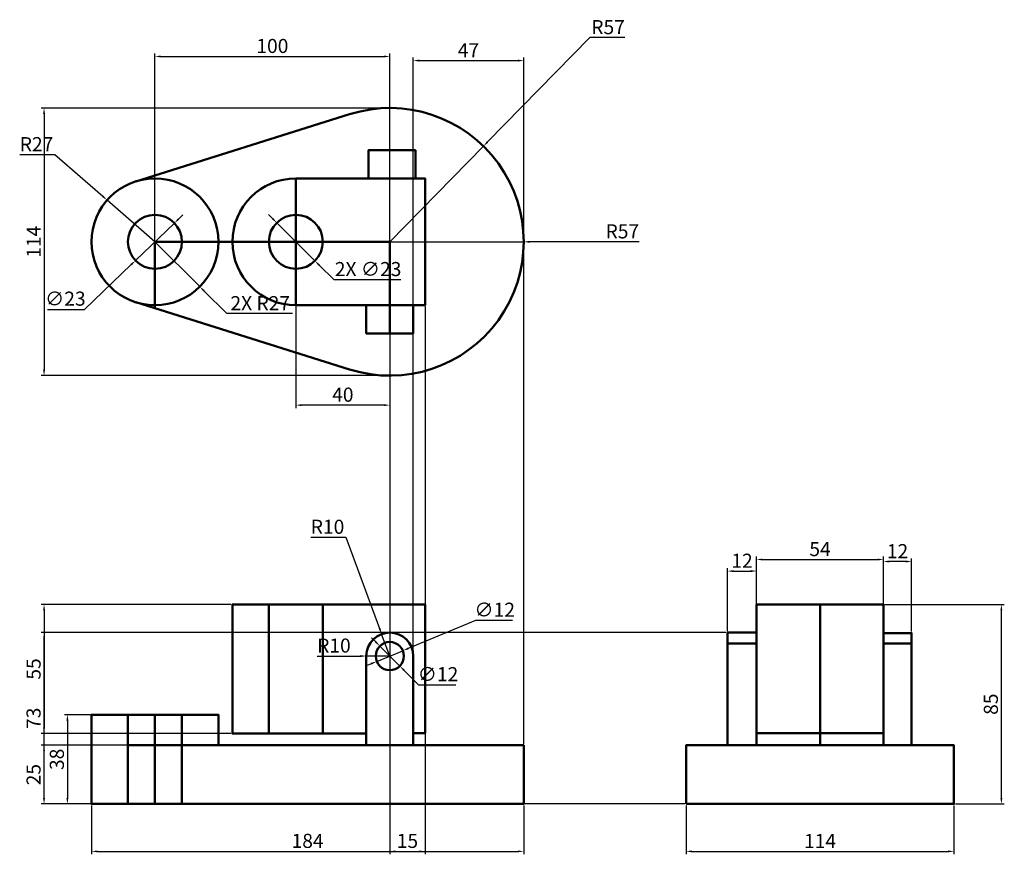
# Model space of a CAD drawing. Units: millimetres. Extents: x 186 to 605, y 16 to 372.
import ezdxf

# ---------------------------------------------------------------- set-up
doc = ezdxf.new("R2010")
doc.units = ezdxf.units.MM
doc.linetypes.add('CENTER', pattern=[50.8, 31.75, -6.35, 6.35, -6.35])
for name, color, linetype, lineweight in [('M-CNTR', 1, 'CENTER', 18), ('M-DIMS', 2, 'Continuous', 25), ('M-OUTL', 7, 'Continuous', 50)]:
    doc.layers.add(name, color=color, linetype=linetype, lineweight=lineweight)
doc.styles.get("Standard").update_dxf_attribs({"font": 'arial.ttf'})
doc.dimstyles.new('ISO-25', dxfattribs={"dimtxt": 6, "dimasz": 2.5, "dimexe": 1.25, "dimexo": 0.625, "dimtad": 1, "dimtoh": 1, "dimdec": 0, "dimtxsty": 'Standard', "dimcen": 2.5, "dimadec": 0, "dimazin": 0, "dimtfac": 1, "dimtdec": 0, "dimtmove": 0, "dimatfit": 3, "dimfxl": 1, "dimarcsym": 0})

# ---------------------------------------------------------------- blocks, each defined once
blk = doc.blocks.new('*D1')
at = {"layer": 'Defpoints', "color": 0, "transparency": 16777216}
for p in [(382.96, 318), (343.1, 277.26)]:
    blk.add_point(p, dxfattribs=at)
at = {"layer": 'M-DIMS', "color": 0, "lineweight": -2, "transparency": 16777216}
for p, q in [((428.23, 364.27), (384.71, 319.79)), ((443.19, 364.27), (428.23, 364.27)), ((343.1, 277.26), (382.96, 318))]:
    blk.add_line(p, q, dxfattribs=at)
at = {"layer": 'M-DIMS', "color": 0, "transparency": 16777216}
blk.add_solid([(384.41, 320.08), (385.01, 319.5), (382.96, 318)], dxfattribs=at)
at = {"layer": 'M-DIMS', "color": 0, "transparency": 16777216, "insert": (436.02, 367.94), "char_height": 6, "attachment_point": 5}
blk.add_mtext('R57', dxfattribs=at)
blk = doc.blocks.new('*D2')
at = {"layer": 'Defpoints', "color": 0, "transparency": 16777216}
for p in [(303.1, 277.26), (343.1, 277.26), (303.1, 207.7)]:
    blk.add_point(p, dxfattribs=at)
at = {"layer": 'M-DIMS', "color": 0, "lineweight": -2, "transparency": 16777216}
for p, q in [((303.1, 276.64), (303.1, 206.45)), ((343.1, 276.64), (343.1, 206.45)), ((340.6, 207.7), (305.6, 207.7))]:
    blk.add_line(p, q, dxfattribs=at)
at = {"layer": 'M-DIMS', "color": 0, "transparency": 16777216}
for points in [[(305.6, 208.12), (305.6, 207.28), (303.1, 207.7)], [(340.6, 208.12), (340.6, 207.28), (343.1, 207.7)]]:
    blk.add_solid(points, dxfattribs=at)
at = {"layer": 'M-DIMS', "color": 0, "transparency": 16777216, "insert": (323.1, 211.39), "char_height": 6, "attachment_point": 5}
blk.add_mtext('40', dxfattribs=at)
blk = doc.blocks.new('*D3')
at = {"layer": 'Defpoints', "color": 0, "transparency": 16777216}
for p in [(343.1, 356.22), (243.1, 277.26), (343.1, 277.26)]:
    blk.add_point(p, dxfattribs=at)
at = {"layer": 'M-DIMS', "color": 0, "lineweight": -2, "transparency": 16777216}
for p, q in [((243.1, 277.89), (243.1, 357.47)), ((343.1, 277.89), (343.1, 357.47)), ((245.6, 356.22), (340.6, 356.22))]:
    blk.add_line(p, q, dxfattribs=at)
at = {"layer": 'M-DIMS', "color": 0, "transparency": 16777216}
for points in [[(245.6, 356.64), (245.6, 355.8), (243.1, 356.22)], [(340.6, 356.64), (340.6, 355.8), (343.1, 356.22)]]:
    blk.add_solid(points, dxfattribs=at)
at = {"layer": 'M-DIMS', "color": 0, "transparency": 16777216, "insert": (293.1, 359.91), "char_height": 6, "attachment_point": 5}
blk.add_mtext('100', dxfattribs=at)
blk = doc.blocks.new('*D4')
at = {"layer": 'Defpoints', "color": 0, "transparency": 16777216}
for p in [(222.75, 295.01), (243.1, 277.26)]:
    blk.add_point(p, dxfattribs=at)
at = {"layer": 'M-DIMS', "color": 0, "lineweight": -2, "transparency": 16777216}
for p, q in [((185.53, 314.44), (200.49, 314.44)), ((200.49, 314.44), (220.87, 296.66)), ((243.1, 277.26), (222.75, 295.01))]:
    blk.add_line(p, q, dxfattribs=at)
at = {"layer": 'M-DIMS', "color": 0, "transparency": 16777216}
blk.add_solid([(221.14, 296.97), (220.6, 296.34), (222.75, 295.01)], dxfattribs=at)
at = {"layer": 'M-DIMS', "color": 0, "transparency": 16777216, "insert": (192.7, 318.08), "char_height": 6, "attachment_point": 5}
blk.add_mtext('R27', dxfattribs=at)
blk = doc.blocks.new('*D5')
at = {"layer": 'Defpoints', "color": 0, "transparency": 16777216}
for p in [(251.38, 285.24), (234.81, 269.29)]:
    blk.add_point(p, dxfattribs=at)
at = {"layer": 'M-DIMS', "color": 0, "lineweight": -2, "transparency": 16777216}
for p, q in [((251.38, 285.24), (234.81, 269.29)), ((253.18, 286.97), (254.99, 288.7)), ((213.14, 248.43), (233.01, 267.55)), ((197.39, 248.43), (213.14, 248.43))]:
    blk.add_line(p, q, dxfattribs=at)
at = {"layer": 'M-DIMS', "color": 0, "transparency": 16777216}
for points in [[(252.9, 287.27), (253.47, 286.67), (251.38, 285.24)], [(232.72, 267.85), (233.3, 267.25), (234.81, 269.29)]]:
    blk.add_solid(points, dxfattribs=at)
at = {"layer": 'M-DIMS', "color": 0, "transparency": 16777216, "insert": (204.96, 252.28), "char_height": 6, "attachment_point": 5}
blk.add_mtext('∅23', dxfattribs=at)
blk = doc.blocks.new('*D6')
at = {"layer": 'Defpoints', "color": 0, "transparency": 16777216}
for p in [(348.64, 103.1), (337.55, 98.51)]:
    blk.add_point(p, dxfattribs=at)
at = {"layer": 'M-DIMS', "color": 0, "lineweight": -2, "transparency": 16777216}
for p, q in [((379.59, 115.93), (350.95, 104.06)), ((395.28, 115.93), (379.59, 115.93)), ((337.55, 98.51), (348.64, 103.1)), ((335.24, 97.56), (332.93, 96.6))]:
    blk.add_line(p, q, dxfattribs=at)
at = {"layer": 'M-DIMS', "color": 0, "transparency": 16777216}
for points in [[(350.79, 104.45), (351.11, 103.68), (348.64, 103.1)], [(335.09, 97.94), (335.4, 97.17), (337.55, 98.51)]]:
    blk.add_solid(points, dxfattribs=at)
at = {"layer": 'M-DIMS', "color": 0, "transparency": 16777216, "insert": (387.75, 119.78), "char_height": 6, "attachment_point": 5}
blk.add_mtext('∅12', dxfattribs=at)
blk = doc.blocks.new('*D7')
at = {"layer": 'Defpoints', "color": 0, "transparency": 16777216}
for p in [(339.63, 110.19), (343.1, 100.81)]:
    blk.add_point(p, dxfattribs=at)
at = {"layer": 'M-DIMS', "color": 0, "lineweight": -2, "transparency": 16777216}
for p, q in [((309.43, 151.42), (324.37, 151.42)), ((324.37, 151.42), (338.76, 112.53)), ((343.1, 100.81), (339.63, 110.19))]:
    blk.add_line(p, q, dxfattribs=at)
at = {"layer": 'M-DIMS', "color": 0, "transparency": 16777216}
blk.add_solid([(339.15, 112.68), (338.37, 112.39), (339.63, 110.19)], dxfattribs=at)
at = {"layer": 'M-DIMS', "color": 0, "transparency": 16777216, "insert": (316.59, 155.11), "char_height": 6, "attachment_point": 5}
blk.add_mtext('R10', dxfattribs=at)
blk = doc.blocks.new('*D8')
at = {"layer": 'Defpoints', "color": 0, "transparency": 16777216}
for p in [(216.1, 75.81), (205.83, 37.81), (216.1, 37.81)]:
    blk.add_point(p, dxfattribs=at)
at = {"layer": 'M-DIMS', "color": 0, "lineweight": -2, "transparency": 16777216}
for p, q in [((215.47, 75.81), (204.58, 75.81)), ((205.83, 73.31), (205.83, 40.31)), ((215.47, 37.81), (204.58, 37.81))]:
    blk.add_line(p, q, dxfattribs=at)
at = {"layer": 'M-DIMS', "color": 0, "transparency": 16777216}
for points in [[(205.41, 73.31), (206.25, 73.31), (205.83, 75.81)], [(205.41, 40.31), (206.25, 40.31), (205.83, 37.81)]]:
    blk.add_solid(points, dxfattribs=at)
at = {"layer": 'M-DIMS', "color": 0, "transparency": 16777216, "insert": (202.14, 56.81), "char_height": 6, "attachment_point": 5, "rotation": 90}
blk.add_mtext('38', dxfattribs=at)
blk = doc.blocks.new('*D9')
at = {"layer": 'Defpoints', "color": 0, "transparency": 16777216}
for p in [(499.25, 137.01), (486.84, 110.81), (499.25, 110.81)]:
    blk.add_point(p, dxfattribs=at)
at = {"layer": 'M-DIMS', "color": 0, "lineweight": -2, "transparency": 16777216}
for p, q in [((486.84, 111.43), (486.84, 138.26)), ((489.34, 137.01), (496.75, 137.01)), ((499.25, 111.43), (499.25, 138.26))]:
    blk.add_line(p, q, dxfattribs=at)
at = {"layer": 'M-DIMS', "color": 0, "transparency": 16777216}
for points in [[(489.34, 137.43), (489.34, 136.6), (486.84, 137.01)], [(496.75, 137.43), (496.75, 136.6), (499.25, 137.01)]]:
    blk.add_solid(points, dxfattribs=at)
at = {"layer": 'M-DIMS', "color": 0, "transparency": 16777216, "insert": (493.05, 140.65), "char_height": 6, "attachment_point": 5}
blk.add_mtext('12', dxfattribs=at)
blk = doc.blocks.new('*D10')
at = {"layer": 'Defpoints', "color": 0, "transparency": 16777216}
for p in [(553.25, 141.93), (499.25, 122.81), (553.25, 122.81)]:
    blk.add_point(p, dxfattribs=at)
at = {"layer": 'M-DIMS', "color": 0, "lineweight": -2, "transparency": 16777216}
for p, q in [((499.25, 123.43), (499.25, 143.18)), ((553.25, 123.43), (553.25, 143.18)), ((501.75, 141.93), (550.75, 141.93))]:
    blk.add_line(p, q, dxfattribs=at)
at = {"layer": 'M-DIMS', "color": 0, "transparency": 16777216}
for points in [[(501.75, 142.35), (501.75, 141.52), (499.25, 141.93)], [(550.75, 142.35), (550.75, 141.52), (553.25, 141.93)]]:
    blk.add_solid(points, dxfattribs=at)
at = {"layer": 'M-DIMS', "color": 0, "transparency": 16777216, "insert": (526.25, 145.61), "char_height": 6, "attachment_point": 5}
blk.add_mtext('54', dxfattribs=at)
blk = doc.blocks.new('*D11')
at = {"layer": 'Defpoints', "color": 0, "transparency": 16777216}
for p in [(553.25, 141.09), (553.25, 110.58), (565.25, 110.58)]:
    blk.add_point(p, dxfattribs=at)
at = {"layer": 'M-DIMS', "color": 0, "lineweight": -2, "transparency": 16777216}
for p, q in [((553.25, 111.2), (553.25, 142.34)), ((562.75, 141.09), (555.75, 141.09)), ((565.25, 111.2), (565.25, 142.34))]:
    blk.add_line(p, q, dxfattribs=at)
at = {"layer": 'M-DIMS', "color": 0, "transparency": 16777216}
for points in [[(555.75, 141.5), (555.75, 140.67), (553.25, 141.09)], [(562.75, 141.5), (562.75, 140.67), (565.25, 141.09)]]:
    blk.add_solid(points, dxfattribs=at)
at = {"layer": 'M-DIMS', "color": 0, "transparency": 16777216, "insert": (559.25, 144.72), "char_height": 6, "attachment_point": 5}
blk.add_mtext('12', dxfattribs=at)
blk = doc.blocks.new('*D12')
at = {"layer": 'Defpoints', "color": 0, "transparency": 16777216}
for p in [(216.1, 37.81), (400.1, 37.81), (400.1, 17.61)]:
    blk.add_point(p, dxfattribs=at)
at = {"layer": 'M-DIMS', "color": 0, "lineweight": -2, "transparency": 16777216}
for p, q in [((216.1, 37.18), (216.1, 16.36)), ((400.1, 37.18), (400.1, 16.36)), ((218.6, 17.61), (397.6, 17.61))]:
    blk.add_line(p, q, dxfattribs=at)
at = {"layer": 'M-DIMS', "color": 0, "transparency": 16777216}
for points in [[(218.6, 18.02), (218.6, 17.19), (216.1, 17.61)], [(397.6, 18.02), (397.6, 17.19), (400.1, 17.61)]]:
    blk.add_solid(points, dxfattribs=at)
at = {"layer": 'M-DIMS', "color": 0, "transparency": 16777216, "insert": (308.1, 21.3), "char_height": 6, "attachment_point": 5}
blk.add_mtext('184', dxfattribs=at)
blk = doc.blocks.new('*D13')
at = {"layer": 'Defpoints', "color": 0, "transparency": 16777216}
for p in [(343.75, 334.26), (195.9, 220.26), (343.75, 220.26)]:
    blk.add_point(p, dxfattribs=at)
at = {"layer": 'M-DIMS', "color": 0, "lineweight": -2, "transparency": 16777216}
for p, q in [((343.13, 334.26), (194.65, 334.26)), ((195.9, 331.76), (195.9, 222.76)), ((343.13, 220.26), (194.65, 220.26))]:
    blk.add_line(p, q, dxfattribs=at)
at = {"layer": 'M-DIMS', "color": 0, "transparency": 16777216}
for points in [[(195.48, 331.76), (196.31, 331.76), (195.9, 334.26)], [(195.48, 222.76), (196.31, 222.76), (195.9, 220.26)]]:
    blk.add_solid(points, dxfattribs=at)
at = {"layer": 'M-DIMS', "color": 0, "transparency": 16777216, "insert": (192.26, 277.26), "char_height": 6, "attachment_point": 5, "rotation": 90}
blk.add_mtext('114', dxfattribs=at)
blk = doc.blocks.new('*D14')
at = {"layer": 'Defpoints', "color": 0, "transparency": 16777216}
for p in [(553.25, 122.81), (603.45, 122.81), (583.25, 37.81)]:
    blk.add_point(p, dxfattribs=at)
at = {"layer": 'M-DIMS', "color": 0, "lineweight": -2, "transparency": 16777216}
for p, q in [((553.88, 122.81), (604.7, 122.81)), ((603.45, 40.31), (603.45, 120.31)), ((583.88, 37.81), (604.7, 37.81))]:
    blk.add_line(p, q, dxfattribs=at)
at = {"layer": 'M-DIMS', "color": 0, "transparency": 16777216}
for points in [[(603.04, 120.31), (603.87, 120.31), (603.45, 122.81)], [(603.04, 40.31), (603.87, 40.31), (603.45, 37.81)]]:
    blk.add_solid(points, dxfattribs=at)
at = {"layer": 'M-DIMS', "color": 0, "transparency": 16777216, "insert": (599.76, 80.31), "char_height": 6, "attachment_point": 5, "rotation": 90}
blk.add_mtext('85', dxfattribs=at)
blk = doc.blocks.new('*D15')
at = {"layer": 'Defpoints', "color": 0, "transparency": 16777216}
for p in [(469.25, 37.81), (583.25, 37.81), (583.25, 17.61)]:
    blk.add_point(p, dxfattribs=at)
at = {"layer": 'M-DIMS', "color": 0, "lineweight": -2, "transparency": 16777216}
for p, q in [((469.25, 37.18), (469.25, 16.36)), ((583.25, 37.18), (583.25, 16.36)), ((471.75, 17.61), (580.75, 17.61))]:
    blk.add_line(p, q, dxfattribs=at)
at = {"layer": 'M-DIMS', "color": 0, "transparency": 16777216}
for points in [[(471.75, 18.02), (471.75, 17.19), (469.25, 17.61)], [(580.75, 18.02), (580.75, 17.19), (583.25, 17.61)]]:
    blk.add_solid(points, dxfattribs=at)
at = {"layer": 'M-DIMS', "color": 0, "transparency": 16777216, "insert": (526.25, 21.25), "char_height": 6, "attachment_point": 5}
blk.add_mtext('114', dxfattribs=at)
blk = doc.blocks.new('*D16')
at = {"layer": 'Defpoints', "color": 0, "transparency": 16777216}
for p in [(343.1, 277.26), (358.1, 250.26), (358.1, 17.61)]:
    blk.add_point(p, dxfattribs=at)
at = {"layer": 'M-DIMS', "color": 0, "lineweight": -2, "transparency": 16777216}
for p, q in [((343.1, 276.64), (343.1, 16.36)), ((358.1, 249.64), (358.1, 16.36)), ((345.6, 17.61), (355.6, 17.61))]:
    blk.add_line(p, q, dxfattribs=at)
at = {"layer": 'M-DIMS', "color": 0, "transparency": 16777216}
for points in [[(345.6, 18.02), (345.6, 17.19), (343.1, 17.61)], [(355.6, 18.02), (355.6, 17.19), (358.1, 17.61)]]:
    blk.add_solid(points, dxfattribs=at)
at = {"layer": 'M-DIMS', "color": 0, "transparency": 16777216, "insert": (350.6, 21.3), "char_height": 6, "attachment_point": 5}
blk.add_mtext('15', dxfattribs=at)
blk = doc.blocks.new('*D17')
at = {"layer": 'Defpoints', "color": 0, "transparency": 16777216}
for p in [(195.9, 110.81), (486.84, 110.81), (469.25, 37.81)]:
    blk.add_point(p, dxfattribs=at)
at = {"layer": 'M-DIMS', "color": 0, "lineweight": -2, "transparency": 16777216}
for p, q in [((486.22, 110.81), (194.65, 110.81)), ((195.9, 40.31), (195.9, 108.31)), ((468.63, 37.81), (194.65, 37.81))]:
    blk.add_line(p, q, dxfattribs=at)
at = {"layer": 'M-DIMS', "color": 0, "transparency": 16777216}
for points in [[(195.48, 108.31), (196.31, 108.31), (195.9, 110.81)], [(195.48, 40.31), (196.31, 40.31), (195.9, 37.81)]]:
    blk.add_solid(points, dxfattribs=at)
at = {"layer": 'M-DIMS', "color": 0, "transparency": 16777216, "insert": (192.21, 74.31), "char_height": 6, "attachment_point": 5, "rotation": 90}
blk.add_mtext('73', dxfattribs=at)
blk = doc.blocks.new('*D18')
at = {"layer": 'Defpoints', "color": 0, "transparency": 16777216}
for p in [(400.1, 354.46), (353.1, 62.81), (400.1, 62.81)]:
    blk.add_point(p, dxfattribs=at)
at = {"layer": 'M-DIMS', "color": 0, "lineweight": -2, "transparency": 16777216}
for p, q in [((353.1, 63.43), (353.1, 355.71)), ((355.6, 354.46), (397.6, 354.46)), ((400.1, 63.43), (400.1, 355.71))]:
    blk.add_line(p, q, dxfattribs=at)
at = {"layer": 'M-DIMS', "color": 0, "transparency": 16777216}
for points in [[(355.6, 354.88), (355.6, 354.04), (353.1, 354.46)], [(397.6, 354.88), (397.6, 354.04), (400.1, 354.46)]]:
    blk.add_solid(points, dxfattribs=at)
at = {"layer": 'M-DIMS', "color": 0, "transparency": 16777216, "insert": (376.6, 358.09), "char_height": 6, "attachment_point": 5}
blk.add_mtext('47', dxfattribs=at)
blk = doc.blocks.new('*D19')
at = {"layer": 'Defpoints', "color": 0, "transparency": 16777216}
for p in [(195.9, 62.81), (231.6, 62.81), (216.1, 37.81)]:
    blk.add_point(p, dxfattribs=at)
at = {"layer": 'M-DIMS', "color": 0, "lineweight": -2, "transparency": 16777216}
for p, q in [((230.97, 62.81), (194.65, 62.81)), ((195.9, 40.31), (195.9, 60.31)), ((215.47, 37.81), (194.65, 37.81))]:
    blk.add_line(p, q, dxfattribs=at)
at = {"layer": 'M-DIMS', "color": 0, "transparency": 16777216}
for points in [[(195.48, 60.31), (196.31, 60.31), (195.9, 62.81)], [(195.48, 40.31), (196.31, 40.31), (195.9, 37.81)]]:
    blk.add_solid(points, dxfattribs=at)
at = {"layer": 'M-DIMS', "color": 0, "transparency": 16777216, "insert": (192.21, 50.31), "char_height": 6, "attachment_point": 5, "rotation": 90}
blk.add_mtext('25', dxfattribs=at)
blk = doc.blocks.new('*D20')
at = {"layer": 'Defpoints', "color": 0, "transparency": 16777216}
for p in [(276.1, 122.81), (195.9, 67.81), (276.1, 67.81)]:
    blk.add_point(p, dxfattribs=at)
at = {"layer": 'M-DIMS', "color": 0, "lineweight": -2, "transparency": 16777216}
for p, q in [((275.47, 122.81), (194.65, 122.81)), ((195.9, 120.31), (195.9, 70.31)), ((275.47, 67.81), (194.65, 67.81))]:
    blk.add_line(p, q, dxfattribs=at)
at = {"layer": 'M-DIMS', "color": 0, "transparency": 16777216}
for points in [[(195.48, 120.31), (196.31, 120.31), (195.9, 122.81)], [(195.48, 70.31), (196.31, 70.31), (195.9, 67.81)]]:
    blk.add_solid(points, dxfattribs=at)
at = {"layer": 'M-DIMS', "color": 0, "transparency": 16777216, "insert": (192.22, 95.31), "char_height": 6, "attachment_point": 5, "rotation": 90}
blk.add_mtext('55', dxfattribs=at)
blk = doc.blocks.new('*D21')
at = {"layer": 'Defpoints', "color": 0, "transparency": 16777216}
for p in [(343.1, 277.26), (400.1, 277.26)]:
    blk.add_point(p, dxfattribs=at)
at = {"layer": 'M-DIMS', "color": 0, "lineweight": -2, "transparency": 16777216}
for p, q in [((343.1, 277.26), (400.1, 277.26)), ((434.3, 277.26), (402.6, 277.26)), ((449.26, 277.26), (434.3, 277.26))]:
    blk.add_line(p, q, dxfattribs=at)
at = {"layer": 'M-DIMS', "color": 0, "transparency": 16777216}
blk.add_solid([(402.6, 277.68), (402.6, 276.84), (400.1, 277.26)], dxfattribs=at)
at = {"layer": 'M-DIMS', "color": 0, "transparency": 16777216, "insert": (442.09, 280.94), "char_height": 6, "attachment_point": 5}
blk.add_mtext('R57', dxfattribs=at)
blk = doc.blocks.new('*D22')
at = {"layer": 'Defpoints', "color": 0, "transparency": 16777216}
for p in [(243.1, 277.26), (262.19, 258.17)]:
    blk.add_point(p, dxfattribs=at)
at = {"layer": 'M-DIMS', "color": 0, "lineweight": -2, "transparency": 16777216}
for p, q in [((243.1, 277.26), (262.19, 258.17)), ((273.65, 246.72), (263.96, 256.4)), ((301.6, 246.72), (273.65, 246.72))]:
    blk.add_line(p, q, dxfattribs=at)
at = {"layer": 'M-DIMS', "color": 0, "transparency": 16777216}
blk.add_solid([(264.25, 256.7), (263.66, 256.11), (262.19, 258.17)], dxfattribs=at)
at = {"layer": 'M-DIMS', "color": 0, "transparency": 16777216, "insert": (287.94, 250.35), "char_height": 6, "attachment_point": 5}
blk.add_mtext('2X R27', dxfattribs=at)
blk = doc.blocks.new('*D23')
at = {"layer": 'Defpoints', "color": 0, "transparency": 16777216}
for p in [(294.97, 285.39), (311.23, 269.13)]:
    blk.add_point(p, dxfattribs=at)
at = {"layer": 'M-DIMS', "color": 0, "lineweight": -2, "transparency": 16777216}
for p, q in [((293.2, 287.16), (291.43, 288.93)), ((294.97, 285.39), (311.23, 269.13)), ((319.34, 261.03), (313, 267.36)), ((347.76, 261.03), (319.34, 261.03))]:
    blk.add_line(p, q, dxfattribs=at)
at = {"layer": 'M-DIMS', "color": 0, "transparency": 16777216}
for points in [[(293.49, 287.45), (292.9, 286.86), (294.97, 285.39)], [(313.29, 267.66), (312.7, 267.07), (311.23, 269.13)]]:
    blk.add_solid(points, dxfattribs=at)
at = {"layer": 'M-DIMS', "color": 0, "transparency": 16777216, "insert": (333.86, 264.88), "char_height": 6, "attachment_point": 5}
blk.add_mtext('2X ∅23', dxfattribs=at)
blk = doc.blocks.new('*D24')
at = {"layer": 'Defpoints', "color": 0, "transparency": 16777216}
for p in [(333.1, 100.81), (343.1, 100.81)]:
    blk.add_point(p, dxfattribs=at)
at = {"layer": 'M-DIMS', "color": 0, "lineweight": -2, "transparency": 16777216}
for p, q in [((312.16, 100.81), (327.1, 100.81)), ((327.1, 100.81), (330.6, 100.81)), ((343.1, 100.81), (333.1, 100.81))]:
    blk.add_line(p, q, dxfattribs=at)
at = {"layer": 'M-DIMS', "color": 0, "transparency": 16777216}
blk.add_solid([(330.6, 101.23), (330.6, 100.39), (333.1, 100.81)], dxfattribs=at)
at = {"layer": 'M-DIMS', "color": 0, "transparency": 16777216, "insert": (319.31, 104.5), "char_height": 6, "attachment_point": 5}
blk.add_mtext('R10', dxfattribs=at)
blk = doc.blocks.new('*D25')
at = {"layer": 'Defpoints', "color": 0, "transparency": 16777216}
for p in [(338.85, 105.05), (347.34, 96.57)]:
    blk.add_point(p, dxfattribs=at)
at = {"layer": 'M-DIMS', "color": 0, "lineweight": -2, "transparency": 16777216}
for p, q in [((337.08, 106.82), (335.32, 108.58)), ((338.85, 105.05), (347.34, 96.57)), ((355.45, 88.47), (349.11, 94.8)), ((371.14, 88.47), (355.45, 88.47))]:
    blk.add_line(p, q, dxfattribs=at)
at = {"layer": 'M-DIMS', "color": 0, "transparency": 16777216}
for points in [[(337.38, 107.11), (336.79, 106.52), (338.85, 105.05)], [(349.41, 95.1), (348.82, 94.51), (347.34, 96.57)]]:
    blk.add_solid(points, dxfattribs=at)
at = {"layer": 'M-DIMS', "color": 0, "transparency": 16777216, "insert": (363.61, 92.32), "char_height": 6, "attachment_point": 5}
blk.add_mtext('∅12', dxfattribs=at)

msp = doc.modelspace()

# ---------------------------------------------------------------- linework, layer by layer
at = {"layer": 'M-CNTR'}
msp.add_line((343.1, 277.26), (343.1, 316.26), dxfattribs=at)
at = {"layer": 'M-OUTL'}
for p, q in [((291.6, 122.81), (291.6, 67.81)), ((314.6, 122.81), (314.6, 67.81)), ((526.25, 62.81), (526.25, 122.81)), ((486.84, 106.2), (499.25, 106.2)), ((553.25, 106.2), (565.25, 106.2)), ((231.6, 75.81), (231.6, 37.81)), ((243.1, 75.81), (243.1, 37.81)), ((254.6, 75.81), (254.6, 37.81)), ((499.25, 67.92), (553.25, 67.92))]:
    msp.add_line(p, q, dxfattribs=at)
for points in [[(235, 303.02), (326, 331.64, -1.36277), (326, 222.89), (235, 251.5)], [(303.1, 250.26, -1), (303.1, 304.26), (303.1, 250.26), (343.1, 250.26), (343.1, 277.26), (243.1, 277.26), (243.1, 248.96)], [(333.1, 62.81), (333.1, 100.81, -1), (353.1, 100.81), (353.1, 62.81)]]:
    msp.add_lwpolyline(points, format="xyb", dxfattribs=at)
for points in [[(333.98, 304.26), (333.98, 316.26), (353.98, 316.26), (353.98, 304.26)], [(343.1, 238.26), (343.1, 250.26), (358.1, 250.26), (358.1, 304.26), (343.1, 304.26), (303.1, 304.26)], [(333.1, 250.26), (333.1, 238.26), (343.1, 238.26), (353.1, 238.26), (353.1, 250.26)], [(333.1, 67.81), (276.1, 67.81), (276.1, 122.81), (343.1, 122.81), (358.1, 122.81), (358.1, 67.92), (353.1, 67.92)], [(499.25, 62.81), (499.25, 122.81), (553.25, 122.81), (553.25, 62.81)], [(499.25, 110.81), (490.84, 110.81), (486.84, 110.81), (486.84, 62.81)], [(553.25, 110.58), (565.25, 110.58), (565.25, 62.81)], [(270.1, 62.81), (270.1, 75.81), (216.1, 75.81), (216.1, 37.81), (400.1, 37.81), (400.1, 62.81), (270.1, 62.81), (231.6, 62.81)]]:
    msp.add_lwpolyline(points, dxfattribs=at)
msp.add_lwpolyline([(469.25, 37.81), (469.25, 62.81), (583.25, 62.81), (583.25, 37.81)], close=True, dxfattribs=at)
for centre, radius in [((243.1, 277.26), 27), ((243.1, 277.26), 11.5), ((303.1, 277.26), 11.5), ((343.1, 100.81), 6)]:
    msp.add_circle(centre, radius, dxfattribs=at)

# ---------------------------------------------------------------- dimensions: what is measured, and where the dimension line sits
at = {"layer": 'M-DIMS'}
for center, mpoint, override, picture, middle in [((343.1, 277.26), (382.96, 318), {"dimclrd": 0, "dimclre": 0, "dimclrt": 0}, '*D1', (436.02, 364.27)), ((243.1, 277.26), (222.75, 295.01), {"dimclrd": 0, "dimclre": 0, "dimclrt": 0}, '*D4', (192.7, 314.44)), ((343.1, 277.26), (400.1, 277.26), {"dimdec": 0, "dimlfac": 1, "dimrnd": 0, "dimzin": 0, "dimdsep": 46, "dimlunit": 2}, '*D21', (434.3, 277.26)), ((343.1, 100.81), (339.63, 110.19), {"dimclrd": 0, "dimclre": 0, "dimclrt": 0}, '*D7', (316.59, 151.42)), ((343.1, 100.81), (333.1, 100.81), {"dimdec": 0, "dimlfac": 1, "dimrnd": 0, "dimzin": 0, "dimdsep": 46, "dimlunit": 2}, '*D24', (327.1, 100.81))]:
    dim = msp.add_radius_dim(center=center, mpoint=mpoint, dimstyle='ISO-25', override=override, dxfattribs=at)
    dim.commit()
    dim.dimension.update_dxf_attribs({"geometry": picture, "text_midpoint": middle, "dimtype": 164})
for base, p1, p2, override, picture, middle in [((343.1, 356.22), (243.1, 277.26), (343.1, 277.26), {"dimclrd": 0, "dimclre": 0, "dimclrt": 0}, '*D3', (293.1, 359.91)), ((400.1, 354.46), (353.1, 62.81), (400.1, 62.81), {"dimdec": 0, "dimlfac": 1, "dimrnd": 0, "dimzin": 0, "dimdsep": 46, "dimlunit": 2}, '*D18', (376.6, 358.09)), ((303.1, 207.7), (343.1, 277.26), (303.1, 277.26), {"dimclrd": 0, "dimclre": 0, "dimclrt": 0}, '*D2', (323.1, 211.39)), ((358.1, 17.61), (343.1, 277.26), (358.1, 250.26), {"dimdec": 0, "dimlfac": 1, "dimrnd": 0, "dimzin": 0, "dimdsep": 46, "dimlunit": 2}, '*D16', (350.6, 21.3)), ((553.25, 141.93), (499.25, 122.81), (553.25, 122.81), {"dimclrd": 0, "dimclre": 0, "dimclrt": 0}, '*D10', (526.25, 145.61)), ((553.25, 141.09), (565.25, 110.58), (553.25, 110.58), {"dimclrd": 0, "dimclre": 0, "dimclrt": 0}, '*D11', (559.25, 144.72)), ((499.25, 137.01), (486.84, 110.81), (499.25, 110.81), {"dimclrd": 0, "dimclre": 0, "dimclrt": 0}, '*D9', (493.05, 140.65)), ((400.1, 17.61), (216.1, 37.81), (400.1, 37.81), {"dimdec": 0, "dimlfac": 1, "dimrnd": 0, "dimzin": 0, "dimdsep": 46, "dimlunit": 2}, '*D12', (308.1, 21.3)), ((583.25, 17.61), (469.25, 37.81), (583.25, 37.81), {"dimdec": 0, "dimlfac": 1, "dimrnd": 0, "dimzin": 0, "dimdsep": 46, "dimlunit": 2}, '*D15', (526.25, 21.25))]:
    dim = msp.add_linear_dim(base=base, p1=p1, p2=p2, dimstyle='ISO-25', override=override, dxfattribs=at)
    dim.commit()
    dim.dimension.update_dxf_attribs({"geometry": picture, "text_midpoint": middle})
for base, p1, p2, override, picture, middle in [((195.9, 220.26), (343.75, 334.26), (343.75, 220.26), {"dimdec": 0, "dimlfac": 1, "dimrnd": 0, "dimzin": 0, "dimdsep": 46, "dimlunit": 2}, '*D13', (192.26, 277.26)), ((195.9, 67.81), (276.1, 122.81), (276.1, 67.81), {"dimdec": 0, "dimlfac": 1, "dimrnd": 0, "dimzin": 0, "dimdsep": 46, "dimlunit": 2}, '*D20', (192.22, 95.31)), ((603.45, 122.81), (583.25, 37.81), (553.25, 122.81), {"dimdec": 0, "dimlfac": 1, "dimrnd": 0, "dimzin": 0, "dimdsep": 46, "dimlunit": 2}, '*D14', (599.76, 80.31)), ((195.9, 110.81), (469.25, 37.81), (486.84, 110.81), {"dimdec": 0, "dimlfac": 1, "dimrnd": 0, "dimzin": 0, "dimdsep": 46, "dimlunit": 2}, '*D17', (192.21, 74.31)), ((205.83, 37.81), (216.1, 75.81), (216.1, 37.81), {"dimclrd": 0, "dimclre": 0, "dimclrt": 0}, '*D8', (202.14, 56.81)), ((195.9, 62.81), (216.1, 37.81), (231.6, 62.81), {"dimdec": 0, "dimlfac": 1, "dimrnd": 0, "dimzin": 0, "dimdsep": 46, "dimlunit": 2}, '*D19', (192.21, 50.31))]:
    dim = msp.add_linear_dim(base=base, p1=p1, p2=p2, angle=90, dimstyle='ISO-25', override=override, dxfattribs=at)
    dim.commit()
    dim.dimension.update_dxf_attribs({"geometry": picture, "text_midpoint": middle})
for p1, p2, override, picture, middle in [((251.38, 285.24), (234.81, 269.29), {"dimclrd": 0, "dimclre": 0, "dimclrt": 0}, '*D5', (204.96, 248.43)), ((337.55, 98.51), (348.64, 103.1), {"dimclrd": 0, "dimclre": 0, "dimclrt": 0}, '*D6', (387.75, 115.93)), ((338.85, 105.05), (347.34, 96.57), {"dimdec": 0, "dimlfac": 1, "dimrnd": 0, "dimzin": 0, "dimdsep": 46, "dimlunit": 2}, '*D25', (363.61, 88.47))]:
    dim = msp.add_diameter_dim_2p(p1=p1, p2=p2, dimstyle='ISO-25', override=override, dxfattribs=at)
    dim.commit()
    dim.dimension.update_dxf_attribs({"geometry": picture, "text_midpoint": middle, "dimtype": 163})
dim = msp.add_diameter_dim_2p(p1=(294.97, 285.39), p2=(311.23, 269.13), text='2X <>', dimstyle='ISO-25', override={"dimdec": 0, "dimlfac": 1, "dimrnd": 0, "dimzin": 0, "dimdsep": 46, "dimlunit": 2}, dxfattribs=at)
dim.commit()
dim.dimension.update_dxf_attribs({"geometry": '*D23', "text_midpoint": (333.86, 261.03), "dimtype": 163})
dim = msp.add_radius_dim(center=(243.1, 277.26), mpoint=(262.19, 258.17), text='2X <>', dimstyle='ISO-25', override={"dimdec": 0, "dimlfac": 1, "dimrnd": 0, "dimzin": 0, "dimdsep": 46, "dimlunit": 2}, dxfattribs=at)
dim.commit()
dim.dimension.update_dxf_attribs({"geometry": '*D22', "text_midpoint": (287.94, 246.72), "dimtype": 164})

doc.saveas('drawing.dxf')
